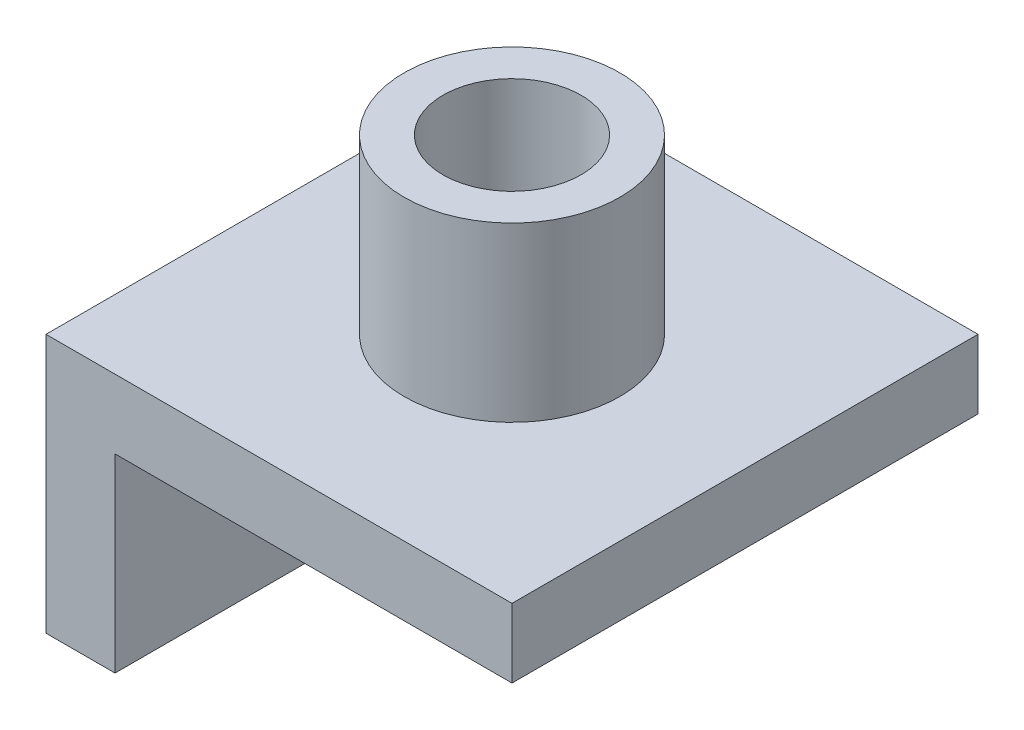
ISO-10303-21;
HEADER;
FILE_DESCRIPTION(('STEP AP214'),'2;1');
FILE_NAME('part.step','',(''),(''),'','','');
FILE_SCHEMA(('AUTOMOTIVE_DESIGN { 1 0 10303 214 1 1 1 1 }'));
ENDSEC;
DATA;
#1=APPLICATION_CONTEXT('core data for automotive mechanical design processes');
#2=APPLICATION_PROTOCOL_DEFINITION('international standard','automotive_design',2000,#1);
#3=PRODUCT_CONTEXT('',#1,'mechanical');
#4=PRODUCT('Part','Part','',(#3));
#5=PRODUCT_RELATED_PRODUCT_CATEGORY('part','',(#4));
#6=PRODUCT_DEFINITION_FORMATION('','',#4);
#7=PRODUCT_DEFINITION_CONTEXT('part definition',#1,'design');
#8=PRODUCT_DEFINITION('design','',#6,#7);
#9=PRODUCT_DEFINITION_SHAPE('','',#8);
#10=(LENGTH_UNIT() NAMED_UNIT(*) SI_UNIT(.MILLI.,.METRE.));
#11=(NAMED_UNIT(*) PLANE_ANGLE_UNIT() SI_UNIT($,.RADIAN.));
#12=(NAMED_UNIT(*) SI_UNIT($,.STERADIAN.) SOLID_ANGLE_UNIT());
#13=UNCERTAINTY_MEASURE_WITH_UNIT(LENGTH_MEASURE(1.E-05),#10,'distance_accuracy_value','');
#14=(GEOMETRIC_REPRESENTATION_CONTEXT(3) GLOBAL_UNCERTAINTY_ASSIGNED_CONTEXT((#13)) GLOBAL_UNIT_ASSIGNED_CONTEXT((#10,
#11,#12)) REPRESENTATION_CONTEXT('',''));
#15=CARTESIAN_POINT('',(0.,0.,0.));
#16=DIRECTION('',(0.,0.,1.));
#17=DIRECTION('',(1.,0.,0.));
#18=AXIS2_PLACEMENT_3D('',#15,#16,#17);
#19=CARTESIAN_POINT('',(8.,0.,54.));
#20=DIRECTION('',(0.,1.,0.));
#21=DIRECTION('',(0.,0.,1.));
#22=AXIS2_PLACEMENT_3D('',#19,#20,#21);
#23=PLANE('',#22);
#24=DIRECTION('',(1.,0.,0.));
#25=VECTOR('',#24,1.);
#26=CARTESIAN_POINT('',(8.,0.,0.));
#27=LINE('',#26,#25);
#28=CARTESIAN_POINT('',(0.,0.,0.));
#29=VERTEX_POINT('',#28);
#30=CARTESIAN_POINT('',(8.,0.,0.));
#31=VERTEX_POINT('',#30);
#32=EDGE_CURVE('E134',#29,#31,#27,.T.);
#33=ORIENTED_EDGE('',*,*,#32,.T.);
#34=DIRECTION('',(0.,0.,-1.));
#35=VECTOR('',#34,1.);
#36=CARTESIAN_POINT('',(8.,0.,54.));
#37=LINE('',#36,#35);
#38=CARTESIAN_POINT('',(8.,0.,54.));
#39=VERTEX_POINT('',#38);
#40=EDGE_CURVE('E48',#39,#31,#37,.T.);
#41=ORIENTED_EDGE('',*,*,#40,.F.);
#42=DIRECTION('',(1.,0.,0.));
#43=VECTOR('',#42,1.);
#44=CARTESIAN_POINT('',(8.,0.,54.));
#45=LINE('',#44,#43);
#46=CARTESIAN_POINT('',(0.,0.,54.));
#47=VERTEX_POINT('',#46);
#48=EDGE_CURVE('E145',#47,#39,#45,.T.);
#49=ORIENTED_EDGE('',*,*,#48,.F.);
#50=DIRECTION('',(0.,0.,-1.));
#51=VECTOR('',#50,1.);
#52=CARTESIAN_POINT('',(0.,0.,54.));
#53=LINE('',#52,#51);
#54=EDGE_CURVE('E130',#47,#29,#53,.T.);
#55=ORIENTED_EDGE('',*,*,#54,.T.);
#56=EDGE_LOOP('',(#33,#41,#49,#55));
#57=FACE_BOUND('',#56,.T.);
#58=ADVANCED_FACE('F44',(#57),#23,.F.);
#59=CARTESIAN_POINT('',(8.,22.,54.));
#60=DIRECTION('',(-1.,0.,0.));
#61=DIRECTION('',(0.,0.,1.));
#62=AXIS2_PLACEMENT_3D('',#59,#60,#61);
#63=PLANE('',#62);
#64=CARTESIAN_POINT('',(8.,11.,27.));
#65=DIRECTION('',(1.,0.,0.));
#66=DIRECTION('',(0.,0.,-1.));
#67=AXIS2_PLACEMENT_3D('',#64,#65,#66);
#68=CIRCLE('',#67,6.);
#69=CARTESIAN_POINT('',(8.,11.,21.));
#70=VERTEX_POINT('',#69);
#71=EDGE_CURVE('E169',#70,#70,#68,.T.);
#72=ORIENTED_EDGE('',*,*,#71,.F.);
#73=EDGE_LOOP('',(#72));
#74=FACE_BOUND('',#73,.T.);
#75=DIRECTION('',(0.,1.,0.));
#76=VECTOR('',#75,1.);
#77=CARTESIAN_POINT('',(8.,22.,0.));
#78=LINE('',#77,#76);
#79=CARTESIAN_POINT('',(8.,22.,0.));
#80=VERTEX_POINT('',#79);
#81=EDGE_CURVE('E133',#31,#80,#78,.T.);
#82=ORIENTED_EDGE('',*,*,#81,.T.);
#83=DIRECTION('',(0.,0.,-1.));
#84=VECTOR('',#83,1.);
#85=CARTESIAN_POINT('',(8.,22.,54.));
#86=LINE('',#85,#84);
#87=CARTESIAN_POINT('',(8.,22.,54.));
#88=VERTEX_POINT('',#87);
#89=EDGE_CURVE('E143',#88,#80,#86,.T.);
#90=ORIENTED_EDGE('',*,*,#89,.F.);
#91=DIRECTION('',(0.,1.,0.));
#92=VECTOR('',#91,1.);
#93=CARTESIAN_POINT('',(8.,22.,54.));
#94=LINE('',#93,#92);
#95=EDGE_CURVE('E99',#39,#88,#94,.T.);
#96=ORIENTED_EDGE('',*,*,#95,.F.);
#97=ORIENTED_EDGE('',*,*,#40,.T.);
#98=EDGE_LOOP('',(#82,#90,#96,#97));
#99=FACE_BOUND('',#98,.T.);
#100=ADVANCED_FACE('F148',(#74,#99),#63,.F.);
#101=CARTESIAN_POINT('',(54.,22.,54.));
#102=DIRECTION('',(0.,1.,0.));
#103=DIRECTION('',(0.,0.,1.));
#104=AXIS2_PLACEMENT_3D('',#101,#102,#103);
#105=PLANE('',#104);
#106=DIRECTION('',(1.,0.,0.));
#107=VECTOR('',#106,1.);
#108=CARTESIAN_POINT('',(54.,22.,0.));
#109=LINE('',#108,#107);
#110=CARTESIAN_POINT('',(54.,22.,0.));
#111=VERTEX_POINT('',#110);
#112=EDGE_CURVE('E139',#80,#111,#109,.T.);
#113=ORIENTED_EDGE('',*,*,#112,.T.);
#114=DIRECTION('',(0.,0.,-1.));
#115=VECTOR('',#114,1.);
#116=CARTESIAN_POINT('',(54.,22.,54.));
#117=LINE('',#116,#115);
#118=CARTESIAN_POINT('',(54.,22.,54.));
#119=VERTEX_POINT('',#118);
#120=EDGE_CURVE('E125',#119,#111,#117,.T.);
#121=ORIENTED_EDGE('',*,*,#120,.F.);
#122=DIRECTION('',(1.,0.,0.));
#123=VECTOR('',#122,1.);
#124=CARTESIAN_POINT('',(54.,22.,54.));
#125=LINE('',#124,#123);
#126=EDGE_CURVE('E113',#88,#119,#125,.T.);
#127=ORIENTED_EDGE('',*,*,#126,.F.);
#128=ORIENTED_EDGE('',*,*,#89,.T.);
#129=EDGE_LOOP('',(#113,#121,#127,#128));
#130=FACE_BOUND('',#129,.T.);
#131=ADVANCED_FACE('F157',(#130),#105,.F.);
#132=CARTESIAN_POINT('',(54.,30.,54.));
#133=DIRECTION('',(-1.,0.,0.));
#134=DIRECTION('',(0.,0.,1.));
#135=AXIS2_PLACEMENT_3D('',#132,#133,#134);
#136=PLANE('',#135);
#137=DIRECTION('',(0.,1.,0.));
#138=VECTOR('',#137,1.);
#139=CARTESIAN_POINT('',(54.,30.,0.));
#140=LINE('',#139,#138);
#141=CARTESIAN_POINT('',(54.,30.,0.));
#142=VERTEX_POINT('',#141);
#143=EDGE_CURVE('E122',#111,#142,#140,.T.);
#144=ORIENTED_EDGE('',*,*,#143,.T.);
#145=DIRECTION('',(0.,0.,-1.));
#146=VECTOR('',#145,1.);
#147=CARTESIAN_POINT('',(54.,30.,54.));
#148=LINE('',#147,#146);
#149=CARTESIAN_POINT('',(54.,30.,54.));
#150=VERTEX_POINT('',#149);
#151=EDGE_CURVE('E117',#150,#142,#148,.T.);
#152=ORIENTED_EDGE('',*,*,#151,.F.);
#153=DIRECTION('',(0.,1.,0.));
#154=VECTOR('',#153,1.);
#155=CARTESIAN_POINT('',(54.,30.,54.));
#156=LINE('',#155,#154);
#157=EDGE_CURVE('E110',#119,#150,#156,.T.);
#158=ORIENTED_EDGE('',*,*,#157,.F.);
#159=ORIENTED_EDGE('',*,*,#120,.T.);
#160=EDGE_LOOP('',(#144,#152,#158,#159));
#161=FACE_BOUND('',#160,.T.);
#162=ADVANCED_FACE('F118',(#161),#136,.F.);
#163=CARTESIAN_POINT('',(0.,30.,54.));
#164=DIRECTION('',(0.,-1.,0.));
#165=DIRECTION('',(0.,0.,-1.));
#166=AXIS2_PLACEMENT_3D('',#163,#164,#165);
#167=PLANE('',#166);
#168=CARTESIAN_POINT('',(27.,30.,27.));
#169=DIRECTION('',(0.,1.,0.));
#170=DIRECTION('',(0.,0.,1.));
#171=AXIS2_PLACEMENT_3D('',#168,#169,#170);
#172=CIRCLE('',#171,12.5);
#173=CARTESIAN_POINT('',(27.,30.,39.5));
#174=VERTEX_POINT('',#173);
#175=EDGE_CURVE('E11',#174,#174,#172,.T.);
#176=ORIENTED_EDGE('',*,*,#175,.F.);
#177=EDGE_LOOP('',(#176));
#178=FACE_BOUND('',#177,.T.);
#179=DIRECTION('',(-1.,0.,0.));
#180=VECTOR('',#179,1.);
#181=CARTESIAN_POINT('',(0.,30.,0.));
#182=LINE('',#181,#180);
#183=CARTESIAN_POINT('',(0.,30.,0.));
#184=VERTEX_POINT('',#183);
#185=EDGE_CURVE('E83',#142,#184,#182,.T.);
#186=ORIENTED_EDGE('',*,*,#185,.T.);
#187=DIRECTION('',(0.,0.,-1.));
#188=VECTOR('',#187,1.);
#189=CARTESIAN_POINT('',(0.,30.,54.));
#190=LINE('',#189,#188);
#191=CARTESIAN_POINT('',(0.,30.,54.));
#192=VERTEX_POINT('',#191);
#193=EDGE_CURVE('E124',#192,#184,#190,.T.);
#194=ORIENTED_EDGE('',*,*,#193,.F.);
#195=DIRECTION('',(-1.,0.,0.));
#196=VECTOR('',#195,1.);
#197=CARTESIAN_POINT('',(0.,30.,54.));
#198=LINE('',#197,#196);
#199=EDGE_CURVE('E111',#150,#192,#198,.T.);
#200=ORIENTED_EDGE('',*,*,#199,.F.);
#201=ORIENTED_EDGE('',*,*,#151,.T.);
#202=EDGE_LOOP('',(#186,#194,#200,#201));
#203=FACE_BOUND('',#202,.T.);
#204=ADVANCED_FACE('F123',(#178,#203),#167,.F.);
#205=CARTESIAN_POINT('',(0.,0.,54.));
#206=DIRECTION('',(1.,0.,0.));
#207=DIRECTION('',(0.,0.,-1.));
#208=AXIS2_PLACEMENT_3D('',#205,#206,#207);
#209=PLANE('',#208);
#210=CARTESIAN_POINT('',(0.,11.,27.));
#211=DIRECTION('',(1.,0.,0.));
#212=DIRECTION('',(0.,0.,-1.));
#213=AXIS2_PLACEMENT_3D('',#210,#211,#212);
#214=CIRCLE('',#213,6.);
#215=CARTESIAN_POINT('',(0.,11.,21.));
#216=VERTEX_POINT('',#215);
#217=EDGE_CURVE('E168',#216,#216,#214,.T.);
#218=ORIENTED_EDGE('',*,*,#217,.T.);
#219=EDGE_LOOP('',(#218));
#220=FACE_BOUND('',#219,.T.);
#221=DIRECTION('',(0.,-1.,0.));
#222=VECTOR('',#221,1.);
#223=CARTESIAN_POINT('',(0.,0.,0.));
#224=LINE('',#223,#222);
#225=EDGE_CURVE('E92',#184,#29,#224,.T.);
#226=ORIENTED_EDGE('',*,*,#225,.T.);
#227=ORIENTED_EDGE('',*,*,#54,.F.);
#228=DIRECTION('',(0.,-1.,0.));
#229=VECTOR('',#228,1.);
#230=CARTESIAN_POINT('',(0.,0.,54.));
#231=LINE('',#230,#229);
#232=EDGE_CURVE('E65',#192,#47,#231,.T.);
#233=ORIENTED_EDGE('',*,*,#232,.F.);
#234=ORIENTED_EDGE('',*,*,#193,.T.);
#235=EDGE_LOOP('',(#226,#227,#233,#234));
#236=FACE_BOUND('',#235,.T.);
#237=ADVANCED_FACE('F174',(#220,#236),#209,.F.);
#238=CARTESIAN_POINT('',(0.,0.,54.));
#239=DIRECTION('',(0.,0.,-1.));
#240=DIRECTION('',(-1.,0.,0.));
#241=AXIS2_PLACEMENT_3D('',#238,#239,#240);
#242=PLANE('',#241);
#243=ORIENTED_EDGE('',*,*,#48,.T.);
#244=ORIENTED_EDGE('',*,*,#95,.T.);
#245=ORIENTED_EDGE('',*,*,#126,.T.);
#246=ORIENTED_EDGE('',*,*,#157,.T.);
#247=ORIENTED_EDGE('',*,*,#199,.T.);
#248=ORIENTED_EDGE('',*,*,#232,.T.);
#249=EDGE_LOOP('',(#243,#244,#245,#246,#247,#248));
#250=FACE_BOUND('',#249,.T.);
#251=ADVANCED_FACE('F107',(#250),#242,.F.);
#252=CARTESIAN_POINT('',(0.,0.,0.));
#253=DIRECTION('',(0.,0.,-1.));
#254=DIRECTION('',(-1.,0.,0.));
#255=AXIS2_PLACEMENT_3D('',#252,#253,#254);
#256=PLANE('',#255);
#257=ORIENTED_EDGE('',*,*,#32,.F.);
#258=ORIENTED_EDGE('',*,*,#225,.F.);
#259=ORIENTED_EDGE('',*,*,#185,.F.);
#260=ORIENTED_EDGE('',*,*,#143,.F.);
#261=ORIENTED_EDGE('',*,*,#112,.F.);
#262=ORIENTED_EDGE('',*,*,#81,.F.);
#263=EDGE_LOOP('',(#257,#258,#259,#260,#261,#262));
#264=FACE_BOUND('',#263,.T.);
#265=ADVANCED_FACE('F152',(#264),#256,.T.);
#266=CARTESIAN_POINT('',(27.,50.,27.));
#267=DIRECTION('',(0.,-1.,0.));
#268=DIRECTION('',(0.,0.,-1.));
#269=AXIS2_PLACEMENT_3D('',#266,#267,#268);
#270=CYLINDRICAL_SURFACE('',#269,12.5);
#271=CARTESIAN_POINT('',(27.,50.,27.));
#272=DIRECTION('',(0.,1.,0.));
#273=DIRECTION('',(0.,0.,1.));
#274=AXIS2_PLACEMENT_3D('',#271,#272,#273);
#275=CIRCLE('',#274,12.5);
#276=CARTESIAN_POINT('',(27.,50.,39.5));
#277=VERTEX_POINT('',#276);
#278=EDGE_CURVE('E132',#277,#277,#275,.T.);
#279=ORIENTED_EDGE('',*,*,#278,.F.);
#280=EDGE_LOOP('',(#279));
#281=FACE_BOUND('',#280,.T.);
#282=ORIENTED_EDGE('',*,*,#175,.T.);
#283=EDGE_LOOP('',(#282));
#284=FACE_BOUND('',#283,.T.);
#285=ADVANCED_FACE('F202',(#281,#284),#270,.T.);
#286=CARTESIAN_POINT('',(27.,50.,27.));
#287=DIRECTION('',(0.,1.,0.));
#288=DIRECTION('',(0.,0.,1.));
#289=AXIS2_PLACEMENT_3D('',#286,#287,#288);
#290=PLANE('',#289);
#291=CARTESIAN_POINT('',(27.,50.,27.));
#292=DIRECTION('',(0.,1.,0.));
#293=DIRECTION('',(0.,0.,1.));
#294=AXIS2_PLACEMENT_3D('',#291,#292,#293);
#295=CIRCLE('',#294,8.);
#296=CARTESIAN_POINT('',(27.,50.,35.));
#297=VERTEX_POINT('',#296);
#298=EDGE_CURVE('E161',#297,#297,#295,.T.);
#299=ORIENTED_EDGE('',*,*,#298,.F.);
#300=EDGE_LOOP('',(#299));
#301=FACE_BOUND('',#300,.T.);
#302=ORIENTED_EDGE('',*,*,#278,.T.);
#303=EDGE_LOOP('',(#302));
#304=FACE_BOUND('',#303,.T.);
#305=ADVANCED_FACE('F207',(#301,#304),#290,.T.);
#306=CARTESIAN_POINT('',(27.,31.,27.));
#307=DIRECTION('',(0.,1.,0.));
#308=DIRECTION('',(0.,0.,1.));
#309=AXIS2_PLACEMENT_3D('',#306,#307,#308);
#310=CYLINDRICAL_SURFACE('',#309,8.);
#311=CARTESIAN_POINT('',(27.,31.,27.));
#312=DIRECTION('',(0.,1.,0.));
#313=DIRECTION('',(0.,0.,1.));
#314=AXIS2_PLACEMENT_3D('',#311,#312,#313);
#315=CIRCLE('',#314,8.);
#316=CARTESIAN_POINT('',(27.,31.,35.));
#317=VERTEX_POINT('',#316);
#318=EDGE_CURVE('E162',#317,#317,#315,.T.);
#319=ORIENTED_EDGE('',*,*,#318,.F.);
#320=EDGE_LOOP('',(#319));
#321=FACE_BOUND('',#320,.T.);
#322=ORIENTED_EDGE('',*,*,#298,.T.);
#323=EDGE_LOOP('',(#322));
#324=FACE_BOUND('',#323,.T.);
#325=ADVANCED_FACE('F208',(#321,#324),#310,.F.);
#326=CARTESIAN_POINT('',(27.,31.,27.));
#327=DIRECTION('',(0.,1.,0.));
#328=DIRECTION('',(0.,0.,1.));
#329=AXIS2_PLACEMENT_3D('',#326,#327,#328);
#330=PLANE('',#329);
#331=ORIENTED_EDGE('',*,*,#318,.T.);
#332=EDGE_LOOP('',(#331));
#333=FACE_BOUND('',#332,.T.);
#334=ADVANCED_FACE('F179',(#333),#330,.T.);
#335=CARTESIAN_POINT('',(0.,11.,27.));
#336=DIRECTION('',(1.,0.,0.));
#337=DIRECTION('',(0.,0.,-1.));
#338=AXIS2_PLACEMENT_3D('',#335,#336,#337);
#339=CYLINDRICAL_SURFACE('',#338,6.);
#340=ORIENTED_EDGE('',*,*,#217,.F.);
#341=EDGE_LOOP('',(#340));
#342=FACE_BOUND('',#341,.T.);
#343=ORIENTED_EDGE('',*,*,#71,.T.);
#344=EDGE_LOOP('',(#343));
#345=FACE_BOUND('',#344,.T.);
#346=ADVANCED_FACE('F180',(#342,#345),#339,.F.);
#347=CLOSED_SHELL('',(#58,#100,#131,#162,#204,#237,#251,#265,#285,#305,#325,#334,#346));
#348=MANIFOLD_SOLID_BREP('B2',#347);
#349=ADVANCED_BREP_SHAPE_REPRESENTATION('',(#18,#348),#14);
#350=SHAPE_DEFINITION_REPRESENTATION(#9,#349);
ENDSEC;
END-ISO-10303-21;
